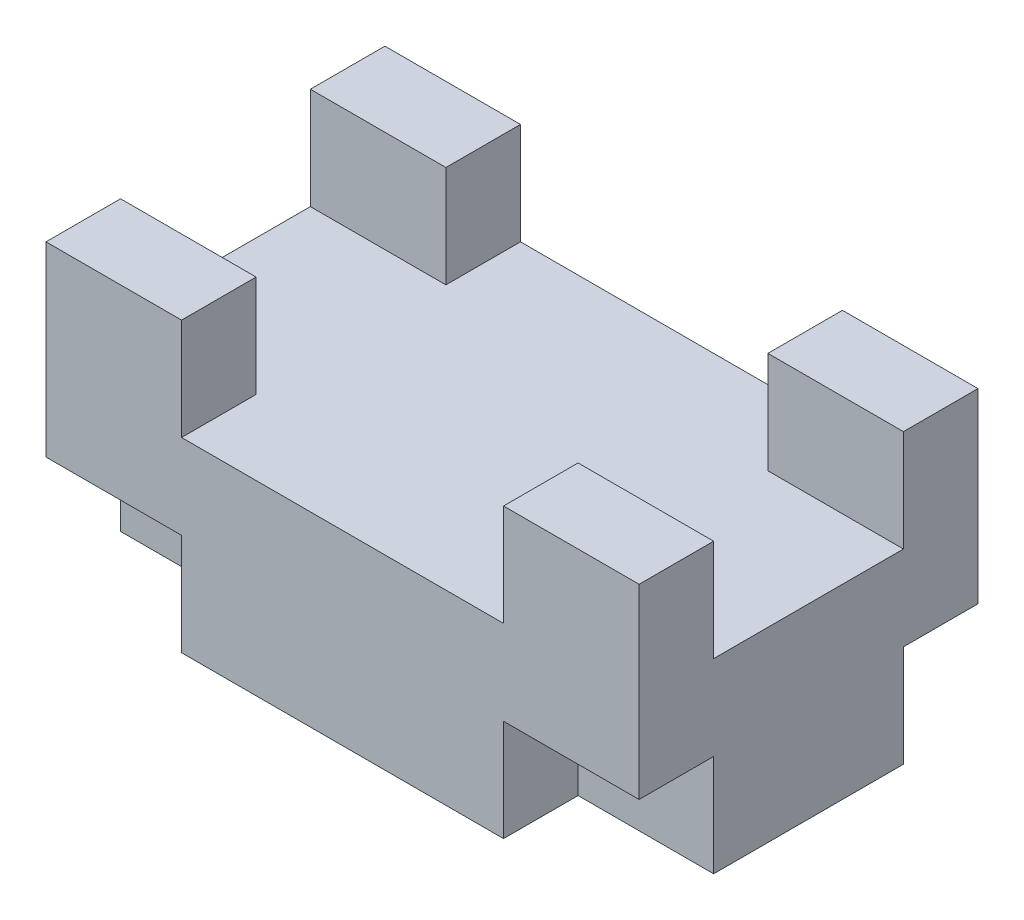
ISO-10303-21;
HEADER;
FILE_DESCRIPTION(('STEP AP214'),'2;1');
FILE_NAME('part.step','',(''),(''),'','','');
FILE_SCHEMA(('AUTOMOTIVE_DESIGN { 1 0 10303 214 1 1 1 1 }'));
ENDSEC;
DATA;
#1=APPLICATION_CONTEXT('core data for automotive mechanical design processes');
#2=APPLICATION_PROTOCOL_DEFINITION('international standard','automotive_design',2000,#1);
#3=PRODUCT_CONTEXT('',#1,'mechanical');
#4=PRODUCT('Part','Part','',(#3));
#5=PRODUCT_RELATED_PRODUCT_CATEGORY('part','',(#4));
#6=PRODUCT_DEFINITION_FORMATION('','',#4);
#7=PRODUCT_DEFINITION_CONTEXT('part definition',#1,'design');
#8=PRODUCT_DEFINITION('design','',#6,#7);
#9=PRODUCT_DEFINITION_SHAPE('','',#8);
#10=(LENGTH_UNIT() NAMED_UNIT(*) SI_UNIT(.MILLI.,.METRE.));
#11=(NAMED_UNIT(*) PLANE_ANGLE_UNIT() SI_UNIT($,.RADIAN.));
#12=(NAMED_UNIT(*) SI_UNIT($,.STERADIAN.) SOLID_ANGLE_UNIT());
#13=UNCERTAINTY_MEASURE_WITH_UNIT(LENGTH_MEASURE(1.E-05),#10,'distance_accuracy_value','');
#14=(GEOMETRIC_REPRESENTATION_CONTEXT(3) GLOBAL_UNCERTAINTY_ASSIGNED_CONTEXT((#13)) GLOBAL_UNIT_ASSIGNED_CONTEXT((#10,
#11,#12)) REPRESENTATION_CONTEXT('',''));
#15=CARTESIAN_POINT('',(0.,0.,0.));
#16=DIRECTION('',(0.,0.,1.));
#17=DIRECTION('',(1.,0.,0.));
#18=AXIS2_PLACEMENT_3D('',#15,#16,#17);
#19=CARTESIAN_POINT('',(0.,0.,0.));
#20=DIRECTION('',(0.,-1.,0.));
#21=DIRECTION('',(0.,0.,-1.));
#22=AXIS2_PLACEMENT_3D('',#19,#20,#21);
#23=PLANE('',#22);
#24=DIRECTION('',(0.,0.,-1.));
#25=VECTOR('',#24,1.);
#26=CARTESIAN_POINT('',(-47.5,0.,-50.));
#27=LINE('',#26,#25);
#28=CARTESIAN_POINT('',(-47.5,0.,-28.));
#29=VERTEX_POINT('',#28);
#30=CARTESIAN_POINT('',(-47.5,0.,-50.));
#31=VERTEX_POINT('',#30);
#32=EDGE_CURVE('E53',#29,#31,#27,.T.);
#33=ORIENTED_EDGE('',*,*,#32,.F.);
#34=DIRECTION('',(1.,0.,0.));
#35=VECTOR('',#34,1.);
#36=CARTESIAN_POINT('',(-87.5,0.,-28.));
#37=LINE('',#36,#35);
#38=CARTESIAN_POINT('',(-87.5,0.,-28.));
#39=VERTEX_POINT('',#38);
#40=EDGE_CURVE('E241',#39,#29,#37,.T.);
#41=ORIENTED_EDGE('',*,*,#40,.F.);
#42=DIRECTION('',(0.,0.,1.));
#43=VECTOR('',#42,1.);
#44=CARTESIAN_POINT('',(-87.5,0.,50.));
#45=LINE('',#44,#43);
#46=CARTESIAN_POINT('',(-87.5,0.,-50.));
#47=VERTEX_POINT('',#46);
#48=EDGE_CURVE('E366',#47,#39,#45,.T.);
#49=ORIENTED_EDGE('',*,*,#48,.F.);
#50=DIRECTION('',(-1.,0.,0.));
#51=VECTOR('',#50,1.);
#52=CARTESIAN_POINT('',(-87.5,0.,-50.));
#53=LINE('',#52,#51);
#54=EDGE_CURVE('E365',#31,#47,#53,.T.);
#55=ORIENTED_EDGE('',*,*,#54,.F.);
#56=EDGE_LOOP('',(#33,#41,#49,#55));
#57=FACE_BOUND('',#56,.T.);
#58=ADVANCED_FACE('F39',(#57),#23,.T.);
#59=DIRECTION('',(-1.,0.,0.));
#60=VECTOR('',#59,1.);
#61=CARTESIAN_POINT('',(-87.5,0.,28.));
#62=LINE('',#61,#60);
#63=CARTESIAN_POINT('',(-47.5,0.,28.));
#64=VERTEX_POINT('',#63);
#65=CARTESIAN_POINT('',(-87.5,0.,28.));
#66=VERTEX_POINT('',#65);
#67=EDGE_CURVE('E64',#64,#66,#62,.T.);
#68=ORIENTED_EDGE('',*,*,#67,.F.);
#69=DIRECTION('',(0.,0.,-1.));
#70=VECTOR('',#69,1.);
#71=CARTESIAN_POINT('',(-47.5,0.,50.));
#72=LINE('',#71,#70);
#73=CARTESIAN_POINT('',(-47.5,0.,50.));
#74=VERTEX_POINT('',#73);
#75=EDGE_CURVE('E386',#74,#64,#72,.T.);
#76=ORIENTED_EDGE('',*,*,#75,.F.);
#77=DIRECTION('',(1.,0.,0.));
#78=VECTOR('',#77,1.);
#79=CARTESIAN_POINT('',(-87.5,0.,50.));
#80=LINE('',#79,#78);
#81=CARTESIAN_POINT('',(-87.5,0.,50.));
#82=VERTEX_POINT('',#81);
#83=EDGE_CURVE('E351',#82,#74,#80,.T.);
#84=ORIENTED_EDGE('',*,*,#83,.F.);
#85=EDGE_CURVE('E370',#66,#82,#45,.T.);
#86=ORIENTED_EDGE('',*,*,#85,.F.);
#87=EDGE_LOOP('',(#68,#76,#84,#86));
#88=FACE_BOUND('',#87,.T.);
#89=ADVANCED_FACE('F484',(#88),#23,.T.);
#90=DIRECTION('',(0.,0.,1.));
#91=VECTOR('',#90,1.);
#92=CARTESIAN_POINT('',(47.5,0.,50.));
#93=LINE('',#92,#91);
#94=CARTESIAN_POINT('',(47.5,0.,28.));
#95=VERTEX_POINT('',#94);
#96=CARTESIAN_POINT('',(47.5,0.,50.));
#97=VERTEX_POINT('',#96);
#98=EDGE_CURVE('E439',#95,#97,#93,.T.);
#99=ORIENTED_EDGE('',*,*,#98,.F.);
#100=DIRECTION('',(-1.,0.,0.));
#101=VECTOR('',#100,1.);
#102=CARTESIAN_POINT('',(87.5,0.,28.));
#103=LINE('',#102,#101);
#104=CARTESIAN_POINT('',(87.5,0.,28.));
#105=VERTEX_POINT('',#104);
#106=EDGE_CURVE('E433',#105,#95,#103,.T.);
#107=ORIENTED_EDGE('',*,*,#106,.F.);
#108=DIRECTION('',(0.,0.,-1.));
#109=VECTOR('',#108,1.);
#110=CARTESIAN_POINT('',(87.5,0.,50.));
#111=LINE('',#110,#109);
#112=CARTESIAN_POINT('',(87.5,0.,50.));
#113=VERTEX_POINT('',#112);
#114=EDGE_CURVE('E363',#113,#105,#111,.T.);
#115=ORIENTED_EDGE('',*,*,#114,.F.);
#116=EDGE_CURVE('E371',#97,#113,#80,.T.);
#117=ORIENTED_EDGE('',*,*,#116,.F.);
#118=EDGE_LOOP('',(#99,#107,#115,#117));
#119=FACE_BOUND('',#118,.T.);
#120=ADVANCED_FACE('F505',(#119),#23,.T.);
#121=CARTESIAN_POINT('',(0.,25.,0.));
#122=DIRECTION('',(0.,-1.,0.));
#123=DIRECTION('',(0.,0.,-1.));
#124=AXIS2_PLACEMENT_3D('',#121,#122,#123);
#125=PLANE('',#124);
#126=DIRECTION('',(0.,0.,1.));
#127=VECTOR('',#126,1.);
#128=CARTESIAN_POINT('',(47.5,25.,50.));
#129=LINE('',#128,#127);
#130=CARTESIAN_POINT('',(47.5,25.,28.));
#131=VERTEX_POINT('',#130);
#132=CARTESIAN_POINT('',(47.5,25.,50.));
#133=VERTEX_POINT('',#132);
#134=EDGE_CURVE('E311',#131,#133,#129,.T.);
#135=ORIENTED_EDGE('',*,*,#134,.F.);
#136=DIRECTION('',(-1.,0.,0.));
#137=VECTOR('',#136,1.);
#138=CARTESIAN_POINT('',(87.5,25.,28.));
#139=LINE('',#138,#137);
#140=CARTESIAN_POINT('',(87.5,25.,28.));
#141=VERTEX_POINT('',#140);
#142=EDGE_CURVE('E290',#141,#131,#139,.T.);
#143=ORIENTED_EDGE('',*,*,#142,.F.);
#144=DIRECTION('',(0.,0.,-1.));
#145=VECTOR('',#144,1.);
#146=CARTESIAN_POINT('',(87.5,25.,50.));
#147=LINE('',#146,#145);
#148=CARTESIAN_POINT('',(87.5,25.,-28.));
#149=VERTEX_POINT('',#148);
#150=EDGE_CURVE('E352',#141,#149,#147,.T.);
#151=ORIENTED_EDGE('',*,*,#150,.T.);
#152=DIRECTION('',(1.,0.,0.));
#153=VECTOR('',#152,1.);
#154=CARTESIAN_POINT('',(87.5,25.,-28.));
#155=LINE('',#154,#153);
#156=CARTESIAN_POINT('',(47.5,25.,-28.));
#157=VERTEX_POINT('',#156);
#158=EDGE_CURVE('E294',#157,#149,#155,.T.);
#159=ORIENTED_EDGE('',*,*,#158,.F.);
#160=DIRECTION('',(0.,0.,1.));
#161=VECTOR('',#160,1.);
#162=CARTESIAN_POINT('',(47.5,25.,-50.));
#163=LINE('',#162,#161);
#164=CARTESIAN_POINT('',(47.5,25.,-50.));
#165=VERTEX_POINT('',#164);
#166=EDGE_CURVE('E257',#165,#157,#163,.T.);
#167=ORIENTED_EDGE('',*,*,#166,.F.);
#168=DIRECTION('',(-1.,0.,0.));
#169=VECTOR('',#168,1.);
#170=CARTESIAN_POINT('',(-87.5,25.,-50.));
#171=LINE('',#170,#169);
#172=CARTESIAN_POINT('',(-47.5,25.,-50.));
#173=VERTEX_POINT('',#172);
#174=EDGE_CURVE('E355',#165,#173,#171,.T.);
#175=ORIENTED_EDGE('',*,*,#174,.T.);
#176=DIRECTION('',(0.,0.,-1.));
#177=VECTOR('',#176,1.);
#178=CARTESIAN_POINT('',(-47.5,25.,-50.));
#179=LINE('',#178,#177);
#180=CARTESIAN_POINT('',(-47.5,25.,-28.));
#181=VERTEX_POINT('',#180);
#182=EDGE_CURVE('E270',#181,#173,#179,.T.);
#183=ORIENTED_EDGE('',*,*,#182,.F.);
#184=DIRECTION('',(1.,0.,0.));
#185=VECTOR('',#184,1.);
#186=CARTESIAN_POINT('',(-87.5,25.,-28.));
#187=LINE('',#186,#185);
#188=CARTESIAN_POINT('',(-87.5,25.,-28.));
#189=VERTEX_POINT('',#188);
#190=EDGE_CURVE('E269',#189,#181,#187,.T.);
#191=ORIENTED_EDGE('',*,*,#190,.F.);
#192=DIRECTION('',(0.,0.,1.));
#193=VECTOR('',#192,1.);
#194=CARTESIAN_POINT('',(-87.5,25.,50.));
#195=LINE('',#194,#193);
#196=CARTESIAN_POINT('',(-87.5,25.,28.));
#197=VERTEX_POINT('',#196);
#198=EDGE_CURVE('E358',#189,#197,#195,.T.);
#199=ORIENTED_EDGE('',*,*,#198,.T.);
#200=DIRECTION('',(-1.,0.,0.));
#201=VECTOR('',#200,1.);
#202=CARTESIAN_POINT('',(-87.5,25.,28.));
#203=LINE('',#202,#201);
#204=CARTESIAN_POINT('',(-47.5,25.,28.));
#205=VERTEX_POINT('',#204);
#206=EDGE_CURVE('E332',#205,#197,#203,.T.);
#207=ORIENTED_EDGE('',*,*,#206,.F.);
#208=DIRECTION('',(0.,0.,-1.));
#209=VECTOR('',#208,1.);
#210=CARTESIAN_POINT('',(-47.5,25.,50.));
#211=LINE('',#210,#209);
#212=CARTESIAN_POINT('',(-47.5,25.,50.));
#213=VERTEX_POINT('',#212);
#214=EDGE_CURVE('E273',#213,#205,#211,.T.);
#215=ORIENTED_EDGE('',*,*,#214,.F.);
#216=DIRECTION('',(1.,0.,0.));
#217=VECTOR('',#216,1.);
#218=CARTESIAN_POINT('',(-87.5,25.,50.));
#219=LINE('',#218,#217);
#220=EDGE_CURVE('E356',#213,#133,#219,.T.);
#221=ORIENTED_EDGE('',*,*,#220,.T.);
#222=EDGE_LOOP('',(#135,#143,#151,#159,#167,#175,#183,#191,#199,#207,#215,#221));
#223=FACE_BOUND('',#222,.T.);
#224=ADVANCED_FACE('F519',(#223),#125,.F.);
#225=CARTESIAN_POINT('',(87.5,25.,50.));
#226=DIRECTION('',(-1.,0.,0.));
#227=DIRECTION('',(0.,0.,1.));
#228=AXIS2_PLACEMENT_3D('',#225,#226,#227);
#229=PLANE('',#228);
#230=ORIENTED_EDGE('',*,*,#114,.T.);
#231=DIRECTION('',(0.,1.,0.));
#232=VECTOR('',#231,1.);
#233=CARTESIAN_POINT('',(87.5,-30.,28.));
#234=LINE('',#233,#232);
#235=CARTESIAN_POINT('',(87.5,-30.,28.));
#236=VERTEX_POINT('',#235);
#237=EDGE_CURVE('E415',#236,#105,#234,.T.);
#238=ORIENTED_EDGE('',*,*,#237,.F.);
#239=DIRECTION('',(0.,0.,1.));
#240=VECTOR('',#239,1.);
#241=CARTESIAN_POINT('',(87.5,-30.,28.));
#242=LINE('',#241,#240);
#243=CARTESIAN_POINT('',(87.5,-30.,-28.));
#244=VERTEX_POINT('',#243);
#245=EDGE_CURVE('E468',#244,#236,#242,.T.);
#246=ORIENTED_EDGE('',*,*,#245,.F.);
#247=DIRECTION('',(0.,1.,0.));
#248=VECTOR('',#247,1.);
#249=CARTESIAN_POINT('',(87.5,-30.,-28.));
#250=LINE('',#249,#248);
#251=CARTESIAN_POINT('',(87.5,0.,-28.));
#252=VERTEX_POINT('',#251);
#253=EDGE_CURVE('E412',#244,#252,#250,.T.);
#254=ORIENTED_EDGE('',*,*,#253,.T.);
#255=CARTESIAN_POINT('',(87.5,0.,-50.));
#256=VERTEX_POINT('',#255);
#257=EDGE_CURVE('E348',#252,#256,#111,.T.);
#258=ORIENTED_EDGE('',*,*,#257,.T.);
#259=DIRECTION('',(0.,-1.,0.));
#260=VECTOR('',#259,1.);
#261=CARTESIAN_POINT('',(87.5,25.,-50.));
#262=LINE('',#261,#260);
#263=CARTESIAN_POINT('',(87.5,55.,-50.));
#264=VERTEX_POINT('',#263);
#265=EDGE_CURVE('E11',#264,#256,#262,.T.);
#266=ORIENTED_EDGE('',*,*,#265,.F.);
#267=DIRECTION('',(0.,0.,-1.));
#268=VECTOR('',#267,1.);
#269=CARTESIAN_POINT('',(87.5,55.,-50.));
#270=LINE('',#269,#268);
#271=CARTESIAN_POINT('',(87.5,55.,-28.));
#272=VERTEX_POINT('',#271);
#273=EDGE_CURVE('E299',#272,#264,#270,.T.);
#274=ORIENTED_EDGE('',*,*,#273,.F.);
#275=DIRECTION('',(0.,-1.,0.));
#276=VECTOR('',#275,1.);
#277=CARTESIAN_POINT('',(87.5,55.,-28.));
#278=LINE('',#277,#276);
#279=EDGE_CURVE('E287',#272,#149,#278,.T.);
#280=ORIENTED_EDGE('',*,*,#279,.T.);
#281=ORIENTED_EDGE('',*,*,#150,.F.);
#282=DIRECTION('',(0.,-1.,0.));
#283=VECTOR('',#282,1.);
#284=CARTESIAN_POINT('',(87.5,55.,28.));
#285=LINE('',#284,#283);
#286=CARTESIAN_POINT('',(87.5,55.,28.));
#287=VERTEX_POINT('',#286);
#288=EDGE_CURVE('E250',#287,#141,#285,.T.);
#289=ORIENTED_EDGE('',*,*,#288,.F.);
#290=DIRECTION('',(0.,0.,-1.));
#291=VECTOR('',#290,1.);
#292=CARTESIAN_POINT('',(87.5,55.,50.));
#293=LINE('',#292,#291);
#294=CARTESIAN_POINT('',(87.5,55.,50.));
#295=VERTEX_POINT('',#294);
#296=EDGE_CURVE('E316',#295,#287,#293,.T.);
#297=ORIENTED_EDGE('',*,*,#296,.F.);
#298=DIRECTION('',(0.,-1.,0.));
#299=VECTOR('',#298,1.);
#300=CARTESIAN_POINT('',(87.5,25.,50.));
#301=LINE('',#300,#299);
#302=EDGE_CURVE('E357',#295,#113,#301,.T.);
#303=ORIENTED_EDGE('',*,*,#302,.T.);
#304=EDGE_LOOP('',(#230,#238,#246,#254,#258,#266,#274,#280,#281,#289,#297,#303));
#305=FACE_BOUND('',#304,.T.);
#306=ADVANCED_FACE('F41',(#305),#229,.F.);
#307=CARTESIAN_POINT('',(-87.5,25.,-50.));
#308=DIRECTION('',(0.,0.,1.));
#309=DIRECTION('',(1.,0.,0.));
#310=AXIS2_PLACEMENT_3D('',#307,#308,#309);
#311=PLANE('',#310);
#312=CARTESIAN_POINT('',(47.5,0.,-50.));
#313=VERTEX_POINT('',#312);
#314=EDGE_CURVE('E364',#256,#313,#53,.T.);
#315=ORIENTED_EDGE('',*,*,#314,.T.);
#316=DIRECTION('',(0.,1.,0.));
#317=VECTOR('',#316,1.);
#318=CARTESIAN_POINT('',(47.5,-30.,-50.));
#319=LINE('',#318,#317);
#320=CARTESIAN_POINT('',(47.5,-30.,-50.));
#321=VERTEX_POINT('',#320);
#322=EDGE_CURVE('E233',#321,#313,#319,.T.);
#323=ORIENTED_EDGE('',*,*,#322,.F.);
#324=DIRECTION('',(1.,0.,0.));
#325=VECTOR('',#324,1.);
#326=CARTESIAN_POINT('',(47.5,-30.,-50.));
#327=LINE('',#326,#325);
#328=CARTESIAN_POINT('',(-47.5,-30.,-50.));
#329=VERTEX_POINT('',#328);
#330=EDGE_CURVE('E221',#329,#321,#327,.T.);
#331=ORIENTED_EDGE('',*,*,#330,.F.);
#332=DIRECTION('',(0.,1.,0.));
#333=VECTOR('',#332,1.);
#334=CARTESIAN_POINT('',(-47.5,-30.,-50.));
#335=LINE('',#334,#333);
#336=EDGE_CURVE('E226',#329,#31,#335,.T.);
#337=ORIENTED_EDGE('',*,*,#336,.T.);
#338=ORIENTED_EDGE('',*,*,#54,.T.);
#339=DIRECTION('',(0.,-1.,0.));
#340=VECTOR('',#339,1.);
#341=CARTESIAN_POINT('',(-87.5,25.,-50.));
#342=LINE('',#341,#340);
#343=CARTESIAN_POINT('',(-87.5,55.,-50.));
#344=VERTEX_POINT('',#343);
#345=EDGE_CURVE('E50',#344,#47,#342,.T.);
#346=ORIENTED_EDGE('',*,*,#345,.F.);
#347=DIRECTION('',(-1.,0.,0.));
#348=VECTOR('',#347,1.);
#349=CARTESIAN_POINT('',(-87.5,55.,-50.));
#350=LINE('',#349,#348);
#351=CARTESIAN_POINT('',(-47.5,55.,-50.));
#352=VERTEX_POINT('',#351);
#353=EDGE_CURVE('E266',#352,#344,#350,.T.);
#354=ORIENTED_EDGE('',*,*,#353,.F.);
#355=DIRECTION('',(0.,-1.,0.));
#356=VECTOR('',#355,1.);
#357=CARTESIAN_POINT('',(-47.5,55.,-50.));
#358=LINE('',#357,#356);
#359=EDGE_CURVE('E263',#352,#173,#358,.T.);
#360=ORIENTED_EDGE('',*,*,#359,.T.);
#361=ORIENTED_EDGE('',*,*,#174,.F.);
#362=DIRECTION('',(0.,-1.,0.));
#363=VECTOR('',#362,1.);
#364=CARTESIAN_POINT('',(47.5,55.,-50.));
#365=LINE('',#364,#363);
#366=CARTESIAN_POINT('',(47.5,55.,-50.));
#367=VERTEX_POINT('',#366);
#368=EDGE_CURVE('E285',#367,#165,#365,.T.);
#369=ORIENTED_EDGE('',*,*,#368,.F.);
#370=DIRECTION('',(-1.,0.,0.));
#371=VECTOR('',#370,1.);
#372=CARTESIAN_POINT('',(87.5,55.,-50.));
#373=LINE('',#372,#371);
#374=EDGE_CURVE('E301',#264,#367,#373,.T.);
#375=ORIENTED_EDGE('',*,*,#374,.F.);
#376=ORIENTED_EDGE('',*,*,#265,.T.);
#377=EDGE_LOOP('',(#315,#323,#331,#337,#338,#346,#354,#360,#361,#369,#375,#376));
#378=FACE_BOUND('',#377,.T.);
#379=ADVANCED_FACE('F229',(#378),#311,.F.);
#380=CARTESIAN_POINT('',(-87.5,25.,50.));
#381=DIRECTION('',(1.,0.,0.));
#382=DIRECTION('',(0.,0.,-1.));
#383=AXIS2_PLACEMENT_3D('',#380,#381,#382);
#384=PLANE('',#383);
#385=ORIENTED_EDGE('',*,*,#48,.T.);
#386=DIRECTION('',(0.,1.,0.));
#387=VECTOR('',#386,1.);
#388=CARTESIAN_POINT('',(-87.5,-30.,-28.));
#389=LINE('',#388,#387);
#390=CARTESIAN_POINT('',(-87.5,-30.,-28.));
#391=VERTEX_POINT('',#390);
#392=EDGE_CURVE('E393',#391,#39,#389,.T.);
#393=ORIENTED_EDGE('',*,*,#392,.F.);
#394=DIRECTION('',(0.,0.,-1.));
#395=VECTOR('',#394,1.);
#396=CARTESIAN_POINT('',(-87.5,-30.,-28.));
#397=LINE('',#396,#395);
#398=CARTESIAN_POINT('',(-87.5,-30.,28.));
#399=VERTEX_POINT('',#398);
#400=EDGE_CURVE('E454',#399,#391,#397,.T.);
#401=ORIENTED_EDGE('',*,*,#400,.F.);
#402=DIRECTION('',(0.,1.,0.));
#403=VECTOR('',#402,1.);
#404=CARTESIAN_POINT('',(-87.5,-30.,28.));
#405=LINE('',#404,#403);
#406=EDGE_CURVE('E400',#399,#66,#405,.T.);
#407=ORIENTED_EDGE('',*,*,#406,.T.);
#408=ORIENTED_EDGE('',*,*,#85,.T.);
#409=DIRECTION('',(0.,-1.,0.));
#410=VECTOR('',#409,1.);
#411=CARTESIAN_POINT('',(-87.5,25.,50.));
#412=LINE('',#411,#410);
#413=CARTESIAN_POINT('',(-87.5,55.,50.));
#414=VERTEX_POINT('',#413);
#415=EDGE_CURVE('E376',#414,#82,#412,.T.);
#416=ORIENTED_EDGE('',*,*,#415,.F.);
#417=DIRECTION('',(0.,0.,1.));
#418=VECTOR('',#417,1.);
#419=CARTESIAN_POINT('',(-87.5,55.,50.));
#420=LINE('',#419,#418);
#421=CARTESIAN_POINT('',(-87.5,55.,28.));
#422=VERTEX_POINT('',#421);
#423=EDGE_CURVE('E330',#422,#414,#420,.T.);
#424=ORIENTED_EDGE('',*,*,#423,.F.);
#425=DIRECTION('',(0.,-1.,0.));
#426=VECTOR('',#425,1.);
#427=CARTESIAN_POINT('',(-87.5,55.,28.));
#428=LINE('',#427,#426);
#429=EDGE_CURVE('E339',#422,#197,#428,.T.);
#430=ORIENTED_EDGE('',*,*,#429,.T.);
#431=ORIENTED_EDGE('',*,*,#198,.F.);
#432=DIRECTION('',(0.,-1.,0.));
#433=VECTOR('',#432,1.);
#434=CARTESIAN_POINT('',(-87.5,55.,-28.));
#435=LINE('',#434,#433);
#436=CARTESIAN_POINT('',(-87.5,55.,-28.));
#437=VERTEX_POINT('',#436);
#438=EDGE_CURVE('E258',#437,#189,#435,.T.);
#439=ORIENTED_EDGE('',*,*,#438,.F.);
#440=DIRECTION('',(0.,0.,1.));
#441=VECTOR('',#440,1.);
#442=CARTESIAN_POINT('',(-87.5,55.,-50.));
#443=LINE('',#442,#441);
#444=EDGE_CURVE('E271',#344,#437,#443,.T.);
#445=ORIENTED_EDGE('',*,*,#444,.F.);
#446=ORIENTED_EDGE('',*,*,#345,.T.);
#447=EDGE_LOOP('',(#385,#393,#401,#407,#408,#416,#424,#430,#431,#439,#445,#446));
#448=FACE_BOUND('',#447,.T.);
#449=ADVANCED_FACE('F385',(#448),#384,.F.);
#450=CARTESIAN_POINT('',(-87.5,25.,50.));
#451=DIRECTION('',(0.,0.,-1.));
#452=DIRECTION('',(-1.,0.,0.));
#453=AXIS2_PLACEMENT_3D('',#450,#451,#452);
#454=PLANE('',#453);
#455=ORIENTED_EDGE('',*,*,#83,.T.);
#456=DIRECTION('',(0.,1.,0.));
#457=VECTOR('',#456,1.);
#458=CARTESIAN_POINT('',(-47.5,-30.,50.));
#459=LINE('',#458,#457);
#460=CARTESIAN_POINT('',(-47.5,-30.,50.));
#461=VERTEX_POINT('',#460);
#462=EDGE_CURVE('E401',#461,#74,#459,.T.);
#463=ORIENTED_EDGE('',*,*,#462,.F.);
#464=DIRECTION('',(-1.,0.,0.));
#465=VECTOR('',#464,1.);
#466=CARTESIAN_POINT('',(-47.5,-30.,50.));
#467=LINE('',#466,#465);
#468=CARTESIAN_POINT('',(47.5,-30.,50.));
#469=VERTEX_POINT('',#468);
#470=EDGE_CURVE('E456',#469,#461,#467,.T.);
#471=ORIENTED_EDGE('',*,*,#470,.F.);
#472=DIRECTION('',(0.,1.,0.));
#473=VECTOR('',#472,1.);
#474=CARTESIAN_POINT('',(47.5,-30.,50.));
#475=LINE('',#474,#473);
#476=EDGE_CURVE('E407',#469,#97,#475,.T.);
#477=ORIENTED_EDGE('',*,*,#476,.T.);
#478=ORIENTED_EDGE('',*,*,#116,.T.);
#479=ORIENTED_EDGE('',*,*,#302,.F.);
#480=DIRECTION('',(1.,0.,0.));
#481=VECTOR('',#480,1.);
#482=CARTESIAN_POINT('',(87.5,55.,50.));
#483=LINE('',#482,#481);
#484=CARTESIAN_POINT('',(47.5,55.,50.));
#485=VERTEX_POINT('',#484);
#486=EDGE_CURVE('E315',#485,#295,#483,.T.);
#487=ORIENTED_EDGE('',*,*,#486,.F.);
#488=DIRECTION('',(0.,-1.,0.));
#489=VECTOR('',#488,1.);
#490=CARTESIAN_POINT('',(47.5,55.,50.));
#491=LINE('',#490,#489);
#492=EDGE_CURVE('E310',#485,#133,#491,.T.);
#493=ORIENTED_EDGE('',*,*,#492,.T.);
#494=ORIENTED_EDGE('',*,*,#220,.F.);
#495=DIRECTION('',(0.,-1.,0.));
#496=VECTOR('',#495,1.);
#497=CARTESIAN_POINT('',(-47.5,55.,50.));
#498=LINE('',#497,#496);
#499=CARTESIAN_POINT('',(-47.5,55.,50.));
#500=VERTEX_POINT('',#499);
#501=EDGE_CURVE('E350',#500,#213,#498,.T.);
#502=ORIENTED_EDGE('',*,*,#501,.F.);
#503=DIRECTION('',(1.,0.,0.));
#504=VECTOR('',#503,1.);
#505=CARTESIAN_POINT('',(-87.5,55.,50.));
#506=LINE('',#505,#504);
#507=EDGE_CURVE('E329',#414,#500,#506,.T.);
#508=ORIENTED_EDGE('',*,*,#507,.F.);
#509=ORIENTED_EDGE('',*,*,#415,.T.);
#510=EDGE_LOOP('',(#455,#463,#471,#477,#478,#479,#487,#493,#494,#502,#508,#509));
#511=FACE_BOUND('',#510,.T.);
#512=ADVANCED_FACE('F483',(#511),#454,.F.);
#513=DIRECTION('',(1.,0.,0.));
#514=VECTOR('',#513,1.);
#515=CARTESIAN_POINT('',(87.5,0.,-28.));
#516=LINE('',#515,#514);
#517=CARTESIAN_POINT('',(47.5,0.,-28.));
#518=VERTEX_POINT('',#517);
#519=EDGE_CURVE('E424',#518,#252,#516,.T.);
#520=ORIENTED_EDGE('',*,*,#519,.F.);
#521=DIRECTION('',(0.,0.,1.));
#522=VECTOR('',#521,1.);
#523=CARTESIAN_POINT('',(47.5,0.,-50.));
#524=LINE('',#523,#522);
#525=EDGE_CURVE('E427',#313,#518,#524,.T.);
#526=ORIENTED_EDGE('',*,*,#525,.F.);
#527=ORIENTED_EDGE('',*,*,#314,.F.);
#528=ORIENTED_EDGE('',*,*,#257,.F.);
#529=EDGE_LOOP('',(#520,#526,#527,#528));
#530=FACE_BOUND('',#529,.T.);
#531=ADVANCED_FACE('F499',(#530),#23,.T.);
#532=CARTESIAN_POINT('',(-47.5,55.,50.));
#533=DIRECTION('',(-1.,0.,0.));
#534=DIRECTION('',(0.,0.,1.));
#535=AXIS2_PLACEMENT_3D('',#532,#533,#534);
#536=PLANE('',#535);
#537=ORIENTED_EDGE('',*,*,#214,.T.);
#538=DIRECTION('',(0.,-1.,0.));
#539=VECTOR('',#538,1.);
#540=CARTESIAN_POINT('',(-47.5,55.,28.));
#541=LINE('',#540,#539);
#542=CARTESIAN_POINT('',(-47.5,55.,28.));
#543=VERTEX_POINT('',#542);
#544=EDGE_CURVE('E344',#543,#205,#541,.T.);
#545=ORIENTED_EDGE('',*,*,#544,.F.);
#546=DIRECTION('',(0.,0.,-1.));
#547=VECTOR('',#546,1.);
#548=CARTESIAN_POINT('',(-47.5,55.,50.));
#549=LINE('',#548,#547);
#550=EDGE_CURVE('E334',#500,#543,#549,.T.);
#551=ORIENTED_EDGE('',*,*,#550,.F.);
#552=ORIENTED_EDGE('',*,*,#501,.T.);
#553=EDGE_LOOP('',(#537,#545,#551,#552));
#554=FACE_BOUND('',#553,.T.);
#555=ADVANCED_FACE('F510',(#554),#536,.F.);
#556=CARTESIAN_POINT('',(-87.5,55.,28.));
#557=DIRECTION('',(0.,0.,1.));
#558=DIRECTION('',(1.,0.,0.));
#559=AXIS2_PLACEMENT_3D('',#556,#557,#558);
#560=PLANE('',#559);
#561=ORIENTED_EDGE('',*,*,#206,.T.);
#562=ORIENTED_EDGE('',*,*,#429,.F.);
#563=DIRECTION('',(-1.,0.,0.));
#564=VECTOR('',#563,1.);
#565=CARTESIAN_POINT('',(-87.5,55.,28.));
#566=LINE('',#565,#564);
#567=EDGE_CURVE('E333',#543,#422,#566,.T.);
#568=ORIENTED_EDGE('',*,*,#567,.F.);
#569=ORIENTED_EDGE('',*,*,#544,.T.);
#570=EDGE_LOOP('',(#561,#562,#568,#569));
#571=FACE_BOUND('',#570,.T.);
#572=ADVANCED_FACE('F511',(#571),#560,.F.);
#573=CARTESIAN_POINT('',(0.,55.,0.));
#574=DIRECTION('',(0.,-1.,0.));
#575=DIRECTION('',(0.,0.,-1.));
#576=AXIS2_PLACEMENT_3D('',#573,#574,#575);
#577=PLANE('',#576);
#578=ORIENTED_EDGE('',*,*,#423,.T.);
#579=ORIENTED_EDGE('',*,*,#507,.T.);
#580=ORIENTED_EDGE('',*,*,#550,.T.);
#581=ORIENTED_EDGE('',*,*,#567,.T.);
#582=EDGE_LOOP('',(#578,#579,#580,#581));
#583=FACE_BOUND('',#582,.T.);
#584=ADVANCED_FACE('F554',(#583),#577,.F.);
#585=CARTESIAN_POINT('',(-87.5,55.,-28.));
#586=DIRECTION('',(0.,0.,-1.));
#587=DIRECTION('',(-1.,0.,0.));
#588=AXIS2_PLACEMENT_3D('',#585,#586,#587);
#589=PLANE('',#588);
#590=ORIENTED_EDGE('',*,*,#190,.T.);
#591=DIRECTION('',(0.,-1.,0.));
#592=VECTOR('',#591,1.);
#593=CARTESIAN_POINT('',(-47.5,55.,-28.));
#594=LINE('',#593,#592);
#595=CARTESIAN_POINT('',(-47.5,55.,-28.));
#596=VERTEX_POINT('',#595);
#597=EDGE_CURVE('E259',#596,#181,#594,.T.);
#598=ORIENTED_EDGE('',*,*,#597,.F.);
#599=DIRECTION('',(1.,0.,0.));
#600=VECTOR('',#599,1.);
#601=CARTESIAN_POINT('',(-87.5,55.,-28.));
#602=LINE('',#601,#600);
#603=EDGE_CURVE('E276',#437,#596,#602,.T.);
#604=ORIENTED_EDGE('',*,*,#603,.F.);
#605=ORIENTED_EDGE('',*,*,#438,.T.);
#606=EDGE_LOOP('',(#590,#598,#604,#605));
#607=FACE_BOUND('',#606,.T.);
#608=ADVANCED_FACE('F557',(#607),#589,.F.);
#609=CARTESIAN_POINT('',(-47.5,55.,-50.));
#610=DIRECTION('',(-1.,0.,0.));
#611=DIRECTION('',(0.,0.,1.));
#612=AXIS2_PLACEMENT_3D('',#609,#610,#611);
#613=PLANE('',#612);
#614=ORIENTED_EDGE('',*,*,#182,.T.);
#615=ORIENTED_EDGE('',*,*,#359,.F.);
#616=DIRECTION('',(0.,0.,-1.));
#617=VECTOR('',#616,1.);
#618=CARTESIAN_POINT('',(-47.5,55.,-50.));
#619=LINE('',#618,#617);
#620=EDGE_CURVE('E280',#596,#352,#619,.T.);
#621=ORIENTED_EDGE('',*,*,#620,.F.);
#622=ORIENTED_EDGE('',*,*,#597,.T.);
#623=EDGE_LOOP('',(#614,#615,#621,#622));
#624=FACE_BOUND('',#623,.T.);
#625=ADVANCED_FACE('F578',(#624),#613,.F.);
#626=CARTESIAN_POINT('',(0.,55.,0.));
#627=DIRECTION('',(0.,1.,0.));
#628=DIRECTION('',(0.,0.,1.));
#629=AXIS2_PLACEMENT_3D('',#626,#627,#628);
#630=PLANE('',#629);
#631=ORIENTED_EDGE('',*,*,#444,.T.);
#632=ORIENTED_EDGE('',*,*,#603,.T.);
#633=ORIENTED_EDGE('',*,*,#620,.T.);
#634=ORIENTED_EDGE('',*,*,#353,.T.);
#635=EDGE_LOOP('',(#631,#632,#633,#634));
#636=FACE_BOUND('',#635,.T.);
#637=ADVANCED_FACE('F572',(#636),#630,.T.);
#638=CARTESIAN_POINT('',(47.5,55.,-50.));
#639=DIRECTION('',(1.,0.,0.));
#640=DIRECTION('',(0.,0.,-1.));
#641=AXIS2_PLACEMENT_3D('',#638,#639,#640);
#642=PLANE('',#641);
#643=ORIENTED_EDGE('',*,*,#166,.T.);
#644=DIRECTION('',(0.,-1.,0.));
#645=VECTOR('',#644,1.);
#646=CARTESIAN_POINT('',(47.5,55.,-28.));
#647=LINE('',#646,#645);
#648=CARTESIAN_POINT('',(47.5,55.,-28.));
#649=VERTEX_POINT('',#648);
#650=EDGE_CURVE('E288',#649,#157,#647,.T.);
#651=ORIENTED_EDGE('',*,*,#650,.F.);
#652=DIRECTION('',(0.,0.,1.));
#653=VECTOR('',#652,1.);
#654=CARTESIAN_POINT('',(47.5,55.,-50.));
#655=LINE('',#654,#653);
#656=EDGE_CURVE('E303',#367,#649,#655,.T.);
#657=ORIENTED_EDGE('',*,*,#656,.F.);
#658=ORIENTED_EDGE('',*,*,#368,.T.);
#659=EDGE_LOOP('',(#643,#651,#657,#658));
#660=FACE_BOUND('',#659,.T.);
#661=ADVANCED_FACE('F579',(#660),#642,.F.);
#662=CARTESIAN_POINT('',(87.5,55.,-28.));
#663=DIRECTION('',(0.,0.,-1.));
#664=DIRECTION('',(-1.,0.,0.));
#665=AXIS2_PLACEMENT_3D('',#662,#663,#664);
#666=PLANE('',#665);
#667=ORIENTED_EDGE('',*,*,#158,.T.);
#668=ORIENTED_EDGE('',*,*,#279,.F.);
#669=DIRECTION('',(1.,0.,0.));
#670=VECTOR('',#669,1.);
#671=CARTESIAN_POINT('',(87.5,55.,-28.));
#672=LINE('',#671,#670);
#673=EDGE_CURVE('E291',#649,#272,#672,.T.);
#674=ORIENTED_EDGE('',*,*,#673,.F.);
#675=ORIENTED_EDGE('',*,*,#650,.T.);
#676=EDGE_LOOP('',(#667,#668,#674,#675));
#677=FACE_BOUND('',#676,.T.);
#678=ADVANCED_FACE('F550',(#677),#666,.F.);
#679=CARTESIAN_POINT('',(0.,55.,0.));
#680=DIRECTION('',(0.,-1.,0.));
#681=DIRECTION('',(0.,0.,-1.));
#682=AXIS2_PLACEMENT_3D('',#679,#680,#681);
#683=PLANE('',#682);
#684=ORIENTED_EDGE('',*,*,#273,.T.);
#685=ORIENTED_EDGE('',*,*,#374,.T.);
#686=ORIENTED_EDGE('',*,*,#656,.T.);
#687=ORIENTED_EDGE('',*,*,#673,.T.);
#688=EDGE_LOOP('',(#684,#685,#686,#687));
#689=FACE_BOUND('',#688,.T.);
#690=ADVANCED_FACE('F539',(#689),#683,.F.);
#691=CARTESIAN_POINT('',(87.5,55.,28.));
#692=DIRECTION('',(0.,0.,1.));
#693=DIRECTION('',(1.,0.,0.));
#694=AXIS2_PLACEMENT_3D('',#691,#692,#693);
#695=PLANE('',#694);
#696=ORIENTED_EDGE('',*,*,#142,.T.);
#697=DIRECTION('',(0.,-1.,0.));
#698=VECTOR('',#697,1.);
#699=CARTESIAN_POINT('',(47.5,55.,28.));
#700=LINE('',#699,#698);
#701=CARTESIAN_POINT('',(47.5,55.,28.));
#702=VERTEX_POINT('',#701);
#703=EDGE_CURVE('E247',#702,#131,#700,.T.);
#704=ORIENTED_EDGE('',*,*,#703,.F.);
#705=DIRECTION('',(-1.,0.,0.));
#706=VECTOR('',#705,1.);
#707=CARTESIAN_POINT('',(87.5,55.,28.));
#708=LINE('',#707,#706);
#709=EDGE_CURVE('E323',#287,#702,#708,.T.);
#710=ORIENTED_EDGE('',*,*,#709,.F.);
#711=ORIENTED_EDGE('',*,*,#288,.T.);
#712=EDGE_LOOP('',(#696,#704,#710,#711));
#713=FACE_BOUND('',#712,.T.);
#714=ADVANCED_FACE('F538',(#713),#695,.F.);
#715=CARTESIAN_POINT('',(47.5,55.,50.));
#716=DIRECTION('',(1.,0.,0.));
#717=DIRECTION('',(0.,0.,-1.));
#718=AXIS2_PLACEMENT_3D('',#715,#716,#717);
#719=PLANE('',#718);
#720=ORIENTED_EDGE('',*,*,#134,.T.);
#721=ORIENTED_EDGE('',*,*,#492,.F.);
#722=DIRECTION('',(0.,0.,1.));
#723=VECTOR('',#722,1.);
#724=CARTESIAN_POINT('',(47.5,55.,50.));
#725=LINE('',#724,#723);
#726=EDGE_CURVE('E321',#702,#485,#725,.T.);
#727=ORIENTED_EDGE('',*,*,#726,.F.);
#728=ORIENTED_EDGE('',*,*,#703,.T.);
#729=EDGE_LOOP('',(#720,#721,#727,#728));
#730=FACE_BOUND('',#729,.T.);
#731=ADVANCED_FACE('F536',(#730),#719,.F.);
#732=CARTESIAN_POINT('',(0.,55.,0.));
#733=DIRECTION('',(0.,1.,0.));
#734=DIRECTION('',(0.,0.,1.));
#735=AXIS2_PLACEMENT_3D('',#732,#733,#734);
#736=PLANE('',#735);
#737=ORIENTED_EDGE('',*,*,#296,.T.);
#738=ORIENTED_EDGE('',*,*,#709,.T.);
#739=ORIENTED_EDGE('',*,*,#726,.T.);
#740=ORIENTED_EDGE('',*,*,#486,.T.);
#741=EDGE_LOOP('',(#737,#738,#739,#740));
#742=FACE_BOUND('',#741,.T.);
#743=ADVANCED_FACE('F530',(#742),#736,.T.);
#744=CARTESIAN_POINT('',(-47.5,-30.,-50.));
#745=DIRECTION('',(1.,0.,0.));
#746=DIRECTION('',(0.,0.,-1.));
#747=AXIS2_PLACEMENT_3D('',#744,#745,#746);
#748=PLANE('',#747);
#749=ORIENTED_EDGE('',*,*,#32,.T.);
#750=ORIENTED_EDGE('',*,*,#336,.F.);
#751=DIRECTION('',(0.,0.,-1.));
#752=VECTOR('',#751,1.);
#753=CARTESIAN_POINT('',(-47.5,-30.,-50.));
#754=LINE('',#753,#752);
#755=CARTESIAN_POINT('',(-47.5,-30.,-28.));
#756=VERTEX_POINT('',#755);
#757=EDGE_CURVE('E232',#756,#329,#754,.T.);
#758=ORIENTED_EDGE('',*,*,#757,.F.);
#759=DIRECTION('',(0.,1.,0.));
#760=VECTOR('',#759,1.);
#761=CARTESIAN_POINT('',(-47.5,-30.,-28.));
#762=LINE('',#761,#760);
#763=EDGE_CURVE('E395',#756,#29,#762,.T.);
#764=ORIENTED_EDGE('',*,*,#763,.T.);
#765=EDGE_LOOP('',(#749,#750,#758,#764));
#766=FACE_BOUND('',#765,.T.);
#767=ADVANCED_FACE('F248',(#766),#748,.F.);
#768=CARTESIAN_POINT('',(47.5,-30.,-50.));
#769=DIRECTION('',(-1.,0.,0.));
#770=DIRECTION('',(0.,0.,1.));
#771=AXIS2_PLACEMENT_3D('',#768,#769,#770);
#772=PLANE('',#771);
#773=ORIENTED_EDGE('',*,*,#525,.T.);
#774=DIRECTION('',(0.,1.,0.));
#775=VECTOR('',#774,1.);
#776=CARTESIAN_POINT('',(47.5,-30.,-28.));
#777=LINE('',#776,#775);
#778=CARTESIAN_POINT('',(47.5,-30.,-28.));
#779=VERTEX_POINT('',#778);
#780=EDGE_CURVE('E252',#779,#518,#777,.T.);
#781=ORIENTED_EDGE('',*,*,#780,.F.);
#782=DIRECTION('',(0.,0.,1.));
#783=VECTOR('',#782,1.);
#784=CARTESIAN_POINT('',(47.5,-30.,-50.));
#785=LINE('',#784,#783);
#786=EDGE_CURVE('E234',#321,#779,#785,.T.);
#787=ORIENTED_EDGE('',*,*,#786,.F.);
#788=ORIENTED_EDGE('',*,*,#322,.T.);
#789=EDGE_LOOP('',(#773,#781,#787,#788));
#790=FACE_BOUND('',#789,.T.);
#791=ADVANCED_FACE('F428',(#790),#772,.F.);
#792=CARTESIAN_POINT('',(87.5,-30.,-28.));
#793=DIRECTION('',(0.,0.,1.));
#794=DIRECTION('',(1.,0.,0.));
#795=AXIS2_PLACEMENT_3D('',#792,#793,#794);
#796=PLANE('',#795);
#797=ORIENTED_EDGE('',*,*,#519,.T.);
#798=ORIENTED_EDGE('',*,*,#253,.F.);
#799=DIRECTION('',(1.,0.,0.));
#800=VECTOR('',#799,1.);
#801=CARTESIAN_POINT('',(87.5,-30.,-28.));
#802=LINE('',#801,#800);
#803=EDGE_CURVE('E422',#779,#244,#802,.T.);
#804=ORIENTED_EDGE('',*,*,#803,.F.);
#805=ORIENTED_EDGE('',*,*,#780,.T.);
#806=EDGE_LOOP('',(#797,#798,#804,#805));
#807=FACE_BOUND('',#806,.T.);
#808=ADVANCED_FACE('F425',(#807),#796,.F.);
#809=CARTESIAN_POINT('',(87.5,-30.,28.));
#810=DIRECTION('',(0.,0.,-1.));
#811=DIRECTION('',(-1.,0.,0.));
#812=AXIS2_PLACEMENT_3D('',#809,#810,#811);
#813=PLANE('',#812);
#814=ORIENTED_EDGE('',*,*,#106,.T.);
#815=DIRECTION('',(0.,1.,0.));
#816=VECTOR('',#815,1.);
#817=CARTESIAN_POINT('',(47.5,-30.,28.));
#818=LINE('',#817,#816);
#819=CARTESIAN_POINT('',(47.5,-30.,28.));
#820=VERTEX_POINT('',#819);
#821=EDGE_CURVE('E406',#820,#95,#818,.T.);
#822=ORIENTED_EDGE('',*,*,#821,.F.);
#823=DIRECTION('',(-1.,0.,0.));
#824=VECTOR('',#823,1.);
#825=CARTESIAN_POINT('',(87.5,-30.,28.));
#826=LINE('',#825,#824);
#827=EDGE_CURVE('E461',#236,#820,#826,.T.);
#828=ORIENTED_EDGE('',*,*,#827,.F.);
#829=ORIENTED_EDGE('',*,*,#237,.T.);
#830=EDGE_LOOP('',(#814,#822,#828,#829));
#831=FACE_BOUND('',#830,.T.);
#832=ADVANCED_FACE('F478',(#831),#813,.F.);
#833=CARTESIAN_POINT('',(47.5,-30.,50.));
#834=DIRECTION('',(-1.,0.,0.));
#835=DIRECTION('',(0.,0.,1.));
#836=AXIS2_PLACEMENT_3D('',#833,#834,#835);
#837=PLANE('',#836);
#838=ORIENTED_EDGE('',*,*,#98,.T.);
#839=ORIENTED_EDGE('',*,*,#476,.F.);
#840=DIRECTION('',(0.,0.,1.));
#841=VECTOR('',#840,1.);
#842=CARTESIAN_POINT('',(47.5,-30.,50.));
#843=LINE('',#842,#841);
#844=EDGE_CURVE('E464',#820,#469,#843,.T.);
#845=ORIENTED_EDGE('',*,*,#844,.F.);
#846=ORIENTED_EDGE('',*,*,#821,.T.);
#847=EDGE_LOOP('',(#838,#839,#845,#846));
#848=FACE_BOUND('',#847,.T.);
#849=ADVANCED_FACE('F481',(#848),#837,.F.);
#850=CARTESIAN_POINT('',(-47.5,-30.,50.));
#851=DIRECTION('',(1.,0.,0.));
#852=DIRECTION('',(0.,0.,-1.));
#853=AXIS2_PLACEMENT_3D('',#850,#851,#852);
#854=PLANE('',#853);
#855=ORIENTED_EDGE('',*,*,#75,.T.);
#856=DIRECTION('',(0.,1.,0.));
#857=VECTOR('',#856,1.);
#858=CARTESIAN_POINT('',(-47.5,-30.,28.));
#859=LINE('',#858,#857);
#860=CARTESIAN_POINT('',(-47.5,-30.,28.));
#861=VERTEX_POINT('',#860);
#862=EDGE_CURVE('E397',#861,#64,#859,.T.);
#863=ORIENTED_EDGE('',*,*,#862,.F.);
#864=DIRECTION('',(0.,0.,-1.));
#865=VECTOR('',#864,1.);
#866=CARTESIAN_POINT('',(-47.5,-30.,50.));
#867=LINE('',#866,#865);
#868=EDGE_CURVE('E452',#461,#861,#867,.T.);
#869=ORIENTED_EDGE('',*,*,#868,.F.);
#870=ORIENTED_EDGE('',*,*,#462,.T.);
#871=EDGE_LOOP('',(#855,#863,#869,#870));
#872=FACE_BOUND('',#871,.T.);
#873=ADVANCED_FACE('F441',(#872),#854,.F.);
#874=CARTESIAN_POINT('',(-87.5,-30.,28.));
#875=DIRECTION('',(0.,0.,-1.));
#876=DIRECTION('',(-1.,0.,0.));
#877=AXIS2_PLACEMENT_3D('',#874,#875,#876);
#878=PLANE('',#877);
#879=ORIENTED_EDGE('',*,*,#67,.T.);
#880=ORIENTED_EDGE('',*,*,#406,.F.);
#881=DIRECTION('',(-1.,0.,0.));
#882=VECTOR('',#881,1.);
#883=CARTESIAN_POINT('',(-87.5,-30.,28.));
#884=LINE('',#883,#882);
#885=EDGE_CURVE('E455',#861,#399,#884,.T.);
#886=ORIENTED_EDGE('',*,*,#885,.F.);
#887=ORIENTED_EDGE('',*,*,#862,.T.);
#888=EDGE_LOOP('',(#879,#880,#886,#887));
#889=FACE_BOUND('',#888,.T.);
#890=ADVANCED_FACE('F448',(#889),#878,.F.);
#891=CARTESIAN_POINT('',(-87.5,-30.,-28.));
#892=DIRECTION('',(0.,0.,1.));
#893=DIRECTION('',(1.,0.,0.));
#894=AXIS2_PLACEMENT_3D('',#891,#892,#893);
#895=PLANE('',#894);
#896=ORIENTED_EDGE('',*,*,#40,.T.);
#897=ORIENTED_EDGE('',*,*,#763,.F.);
#898=DIRECTION('',(1.,0.,0.));
#899=VECTOR('',#898,1.);
#900=CARTESIAN_POINT('',(-87.5,-30.,-28.));
#901=LINE('',#900,#899);
#902=EDGE_CURVE('E238',#391,#756,#901,.T.);
#903=ORIENTED_EDGE('',*,*,#902,.F.);
#904=ORIENTED_EDGE('',*,*,#392,.T.);
#905=EDGE_LOOP('',(#896,#897,#903,#904));
#906=FACE_BOUND('',#905,.T.);
#907=ADVANCED_FACE('F490',(#906),#895,.F.);
#908=CARTESIAN_POINT('',(0.,-30.,0.));
#909=DIRECTION('',(0.,1.,0.));
#910=DIRECTION('',(0.,0.,1.));
#911=AXIS2_PLACEMENT_3D('',#908,#909,#910);
#912=PLANE('',#911);
#913=ORIENTED_EDGE('',*,*,#757,.T.);
#914=ORIENTED_EDGE('',*,*,#330,.T.);
#915=ORIENTED_EDGE('',*,*,#786,.T.);
#916=ORIENTED_EDGE('',*,*,#803,.T.);
#917=ORIENTED_EDGE('',*,*,#245,.T.);
#918=ORIENTED_EDGE('',*,*,#827,.T.);
#919=ORIENTED_EDGE('',*,*,#844,.T.);
#920=ORIENTED_EDGE('',*,*,#470,.T.);
#921=ORIENTED_EDGE('',*,*,#868,.T.);
#922=ORIENTED_EDGE('',*,*,#885,.T.);
#923=ORIENTED_EDGE('',*,*,#400,.T.);
#924=ORIENTED_EDGE('',*,*,#902,.T.);
#925=EDGE_LOOP('',(#913,#914,#915,#916,#917,#918,#919,#920,#921,#922,#923,#924));
#926=FACE_BOUND('',#925,.T.);
#927=ADVANCED_FACE('F236',(#926),#912,.F.);
#928=CLOSED_SHELL('',(#58,#89,#120,#224,#306,#379,#449,#512,#531,#555,#572,#584,#608,#625,#637,
#661,#678,#690,#714,#731,#743,#767,#791,#808,#832,#849,#873,#890,#907,#927));
#929=MANIFOLD_SOLID_BREP('B2',#928);
#930=ADVANCED_BREP_SHAPE_REPRESENTATION('',(#18,#929),#14);
#931=SHAPE_DEFINITION_REPRESENTATION(#9,#930);
ENDSEC;
END-ISO-10303-21;
